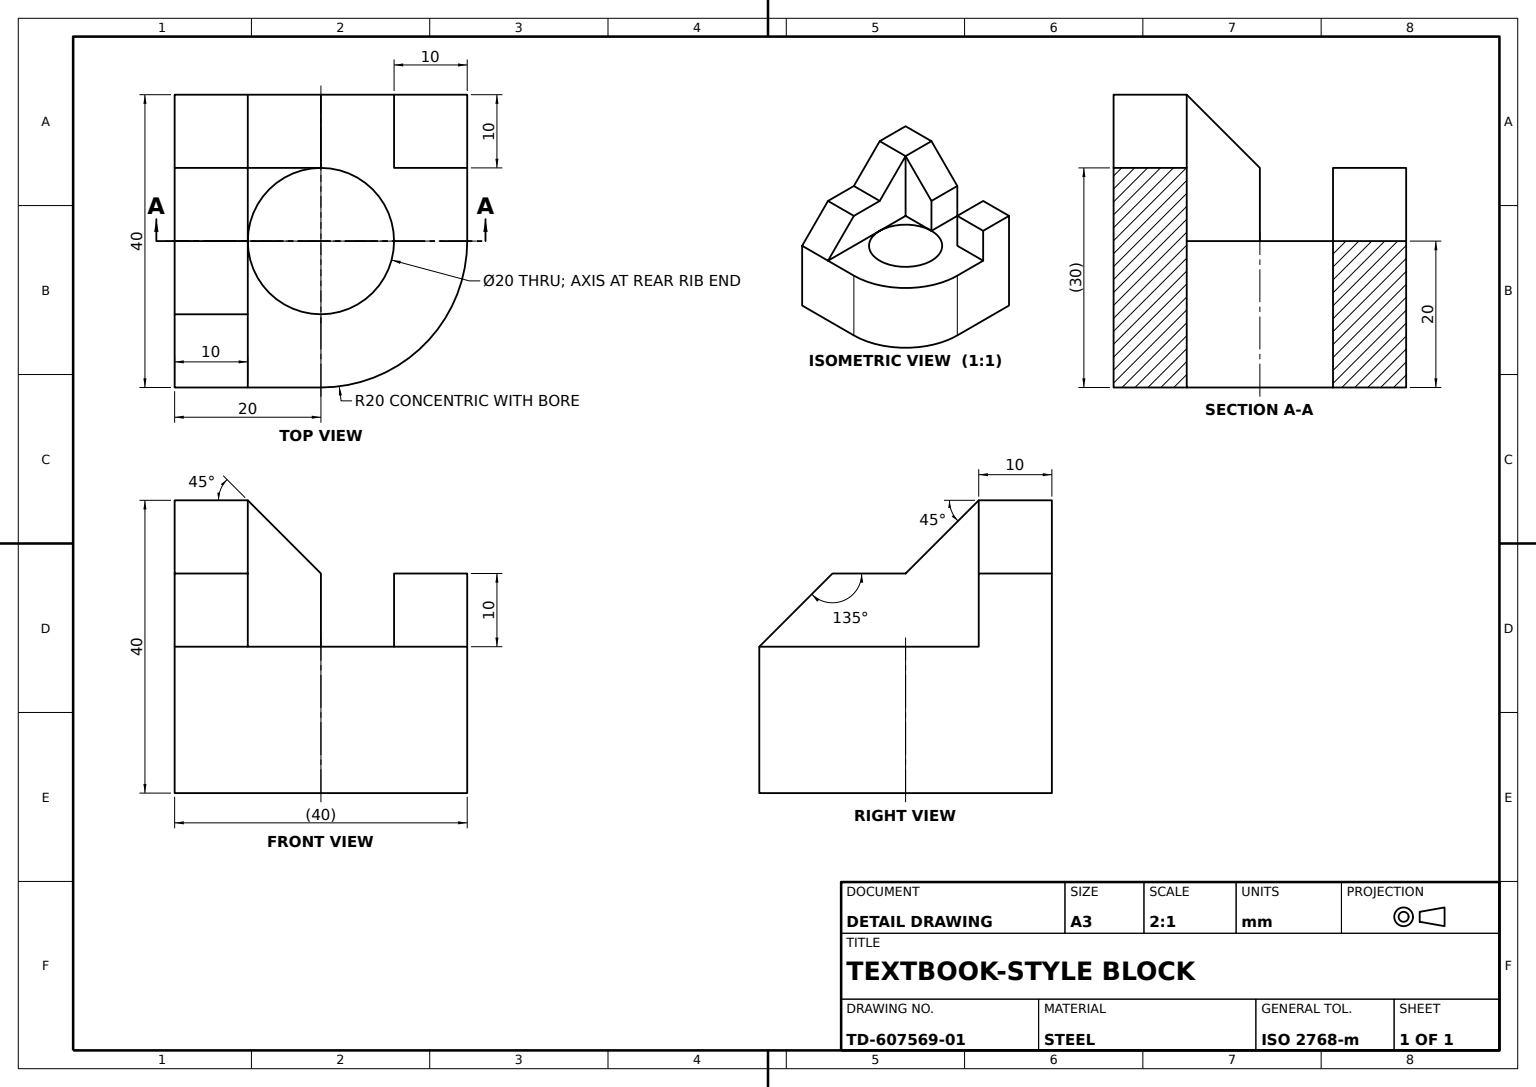
from build123d import *

# Parameters (mm, degrees)
BASE_BLOCK_DEPTH        = 10
CORNER_POST_PROFILE_W   = 10
CORNER_POST_PROFILE_H   = 10
CORNER_POST_10X10_DEPTH = 10
STEPPED_RIB_DEPTH       = 10
GUSSET_DEPTH            = 10
BORE_PROFILE_R          = 10
BORE_20_DEPTH           = 20


with BuildPart() as part:
    # Base Block Profile → Base Block (new, symmetric)
    with BuildSketch(Plane(origin=(0, 0, 0), x_dir=(1, 0, 0), z_dir=(0, 1, 0))):
        with BuildLine():
            Line((0, -20), (-20, -20))
            Line((-20, -20), (-20, 20))
            Line((-20, 20), (20, 20))
            Line((20, 20), (20, 0))
            ThreePointArc((20, 0), (14.142135624, -14.142135624), (0, -20))
        make_face()
    extrude(amount=BASE_BLOCK_DEPTH, both=True)

    # Corner Post Profile → Corner Post 10x10 (add)
    with BuildSketch(Plane(origin=(0, 10, 0), x_dir=(1, 0, 0), z_dir=(0, 1, 0))):
        with Locations((15, 15)):
            Rectangle(CORNER_POST_PROFILE_W, CORNER_POST_PROFILE_H)
    extrude(amount=CORNER_POST_10X10_DEPTH)

    # Stepped Rib Profile → Stepped Rib (add)
    with BuildSketch(Plane.ZY.offset(20)):
        Polygon((-20, 10), (-20, 30), (-10, 30), (0, 20), (10, 20), (20, 10), align=None)
    extrude(amount=-STEPPED_RIB_DEPTH)

    # Gusset Profile → Gusset (add)
    with BuildSketch(Plane(origin=(0, 0, -20), x_dir=(-1, 0, 0), z_dir=(0, 0, -1))):
        Polygon((10, 10), (10, 30), (0, 20), (0, 10), align=None)
    extrude(amount=-GUSSET_DEPTH)

    # Bore Profile → Bore Ø20 (cut)
    with BuildSketch(Plane.XZ.offset(10)):
        with Locations(Location((0, 0, 0), (0, 0, 270))):
            Circle(BORE_PROFILE_R)
    extrude(amount=-BORE_20_DEPTH, mode=Mode.SUBTRACT)


solid = part.part
